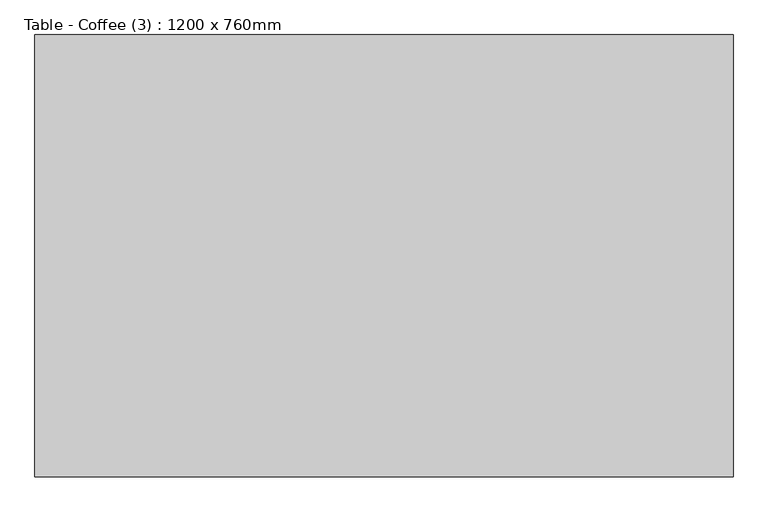
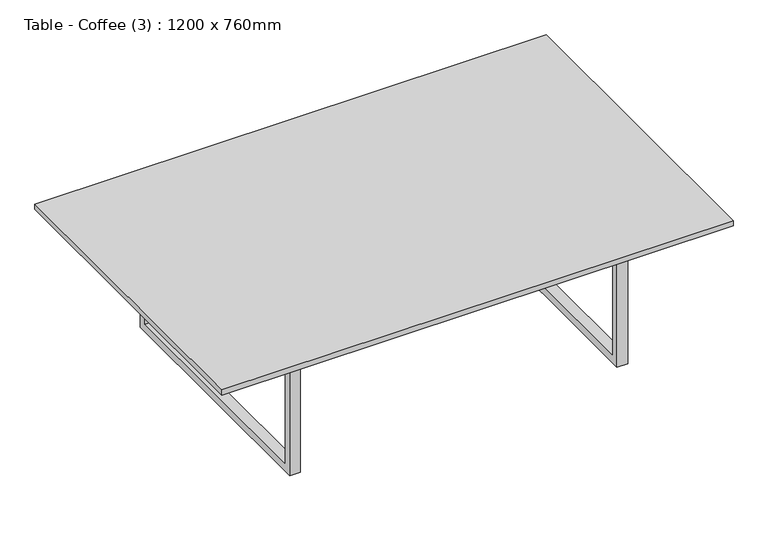
"""IFC4 building model written with IfcOpenShell, lengths in millimetres: furniture geometry, Table - Coffee (3) : 1200 x 760mm."""

from ifc_helpers import new_model, si_unit, frame, origin, place, context, project, spatial, polyline, outline, extrude, source, transform, mapped, element, save


def table_coffee_3_1200_x_760mm_bccf866f(model_context):
    return source(origin(), model_context, "Body", "SweptSolid", [
        extrude(outline(polyline([(1203.7336303, 748.6108318), (1203.7336303, -11.3891682), (3.7336303, -11.3891682), (3.7336303, 748.6108318), (1203.7336303, 748.6108318)])), frame((0.0, 0.0, 317.3), z_axis=(0.0, 0.0, 1.0), x_axis=(1.0, 0.0, 0.0)), (0.0, 0.0, 1.0), 12.7),
        extrude(outline(polyline([(64.8108318, 317.3), (672.4108318, 317.3), (672.4108318, 0.0), (64.8108318, 0.0), (64.8108318, 317.3)]), holes=[polyline([(83.8608318, 298.25), (83.8608318, 19.05), (653.3608318, 19.05), (653.3608318, 298.25), (83.8608318, 298.25)])]), frame((206.9336303, 0.0, 0.0), z_axis=(1.0, 0.0, 0.0), x_axis=(0.0, 1.0, 0.0)), (0.0, 0.0, 1.0), 25.4),
        extrude(outline(polyline([(64.8108318, 317.3), (672.4108318, 317.3), (672.4108318, 0.0), (64.8108318, 0.0), (64.8108318, 317.3)]), holes=[polyline([(83.8608318, 298.25), (83.8608318, 19.05), (653.3608318, 19.05), (653.3608318, 298.25), (83.8608318, 298.25)])]), frame((975.1336303, 0.0, 0.0), z_axis=(1.0, 0.0, 0.0), x_axis=(0.0, 1.0, 0.0)), (0.0, 0.0, 1.0), 25.4),
        extrude(outline(polyline([(975.1336303, 378.1358318), (975.1336303, 359.0858318), (232.3336303, 359.0858318), (232.3336303, 378.1358318), (975.1336303, 378.1358318)])), frame((0.0, 0.0, 298.25), z_axis=(0.0, 0.0, 1.0), x_axis=(1.0, 0.0, 0.0)), (0.0, 0.0, 1.0), 19.05),
    ])


if __name__ == "__main__":
    model = new_model("IFC4")
    model_context = context("Model", 3, world=origin())
    ifc_project = project(units=[si_unit("LENGTHUNIT", "METRE", prefix="MILLI")], contexts=[model_context])
    site = spatial("IfcSite", under=ifc_project)
    building = spatial("IfcBuilding", under=site)
    placement = place(None, origin())
    table_coffee_3_1200_x_760mm_shape = table_coffee_3_1200_x_760mm_bccf866f(model_context)
    element("IfcFurniture", 1, ObjectType="Table - Coffee (3) : 1200 x 760mm", at=placement, inside=building, context=model_context, shape_type="MappedRepresentation", body=[
        mapped(table_coffee_3_1200_x_760mm_shape, transform((0.0, 0.0, 0.0), x_axis=(1.0, 0.0, 0.0), y_axis=(0.0, 1.0, 0.0), z_axis=(0.0, 0.0, 1.0))),
    ])
    save(model, "model.ifc")

# Revit data of these elements
# Type "Table - Coffee (3) : 1200 x 760mm"
#   Keynote = "N"
#   Height = 330 mm
#   Length = 1200 mm
#   Width = 760 mm
#   Material Base = Metal - Chrome
#   Material Top = Glass - Clear, Grey
#   Default Elevation = 0
#   Assembly Code = ""
# Element 1 (IfcFurniture, "Table - Coffee (3) : 1200 x 760mm")
#   Materials on its faces: "Metal - Chrome", "Glass - Clear, Grey"
# Materials
#   "Metal - Chrome": colour RGB 17 17 17, transparency 0
#   "Glass - Clear, Grey": colour RGB 252 255 255, transparency 0.64
